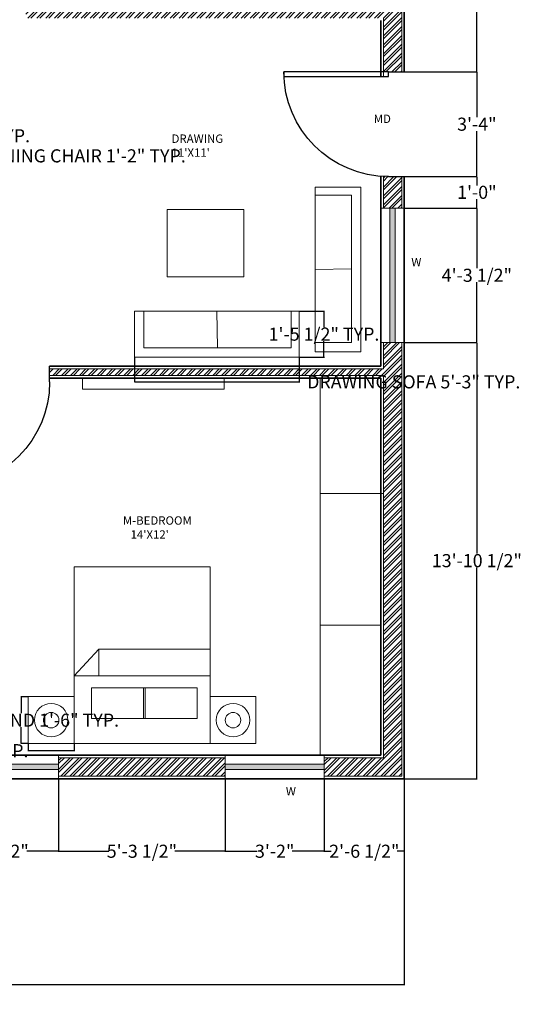
# Model space of a CAD drawing. Units: inches. Extents: x -340 to 394, y 381 to 1380.
# Tile 2 of 3: x 195 to 386, y 381 to 757. Entities that reach past the tile are written whole.
import ezdxf

# ---------------------------------------------------------------- set-up
doc = ezdxf.new("R2010")
doc.units = ezdxf.units.IN
doc.header["$MEASUREMENT"] = 0
for name, color, linetype, lineweight in [('A-ANNO-DIMS', 150, 'Continuous', 18), ('A-ANNO-TEXT', 11, 'Continuous', 18), ('A-AREA-IDEN', 11, 'Continuous', 18), ('A-FLOR-CASE', 130, 'Continuous', 20), ('A-GLAZ-PATT', 220, 'Continuous', 13), ('A-WALL-FNSH', 150, 'Continuous', 18), ('A-WALL-PATT', 10, 'Continuous', 13), ('door', 200, 'Continuous', 25), ('fur', 130, 'Continuous', 18), ('wall', 150, 'Continuous', 35), ('wind', 220, 'Continuous', 20)]:
    doc.layers.add(name, color=color, linetype=linetype, lineweight=lineweight)
doc.styles.get("Standard").update_dxf_attribs({"font": 'arial.ttf'})
doc.dimstyles.get("Standard").update_dxf_attribs({"dimtxt": 5, "dimasz": 0.18, "dimexe": 0.18, "dimexo": 0.0625, "dimgap": 0.09, "dimtad": 0, "dimtih": 1, "dimtoh": 1, "dimdec": 0, "dimzin": 0, "dimdsep": 46, "dimlunit": 4, "dimtxsty": 'Standard', "dimcen": 0.09, "dimadec": 0, "dimazin": 0, "dimtfac": 1, "dimtdec": 0, "dimtofl": 0, "dimtmove": 0, "dimatfit": 3, "dimfxl": 1, "dimtolj": 1, "dimtzin": 0, "dimarcsym": 0})

# ---------------------------------------------------------------- blocks, each defined once
blk = doc.blocks.new('*U2')
for p, q in [((0, 0), (0, -6)), ((40, 0), (40, -6))]:
    blk.add_line(p, q)
blk.add_lwpolyline([(0, 0), (0, 40), (1.75, 40), (1.75, 0)], close=True)
blk.add_arc((0, 0), 40, 0, 90)
blk = doc.blocks.new('BED-DOUBLE')
for p, q in [((25.93, 0), (25.93, 51.94)), ((25.93, 51.94), (25.93, 42.46)), ((36.06, 42.46), (25.93, 51.94)), ((25.93, 51.94), (36.06, 42.46)), ((25.93, 42.46), (36.06, 42.46)), ((36.06, 42.46), (36.06, 0))]:
    blk.add_line(p, q)
for points in [[(0, 0), (67.52, 0), (67.52, 51.94), (0, 51.94)], [(9.57, 24.81), (21.34, 24.81), (21.34, 45.28), (9.57, 45.28)], [(9.57, 4.93), (21.34, 4.93), (21.34, 25.4), (9.57, 25.4)]]:
    blk.add_lwpolyline(points, close=True)
blk = doc.blocks.new('NIGHTSTAND')
blk.add_lwpolyline([(0, 0), (17.94, 0), (17.94, 17.5), (0, 17.5)], close=True)
for radius in [6.39, 2.96]:
    blk.add_circle((8.97, 8.75), radius)
blk = doc.blocks.new('SOFA-DRAWING-ROOM')
for p, q in [((3.53, 17.55), (3.53, 3.6)), ((31.47, 17.55), (31.68, 3.6)), ((59.83, 3.6), (59.83, 17.55)), ((3.53, 3.6), (59.83, 3.6))]:
    blk.add_line(p, q)
blk.add_lwpolyline([(0, 0), (62.94, 0), (62.94, 17.55), (0, 17.55)], close=True)
blk = doc.blocks.new('*D13')
at = {"layer": 'A-ANNO-DIMS', "color": 0, "lineweight": -2, "transparency": 16777216}
for p, q in [((197.74, 498.52), (194.94, 498.52)), ((195.12, 498.34), (195.12, 492.23)), ((195.12, 480.77), (195.12, 486.88)), ((197.74, 480.59), (194.94, 480.59))]:
    blk.add_line(p, q, dxfattribs=at)
at = {"layer": 'A-ANNO-DIMS', "color": 0, "transparency": 16777216}
for points in [[(195.09, 498.34), (195.15, 498.34), (195.12, 498.52)], [(195.09, 480.77), (195.15, 480.77), (195.12, 480.59)]]:
    blk.add_solid(points, dxfattribs=at)
at = {"layer": 'Defpoints', "color": 0, "transparency": 16777216}
for p in [(195.12, 498.52), (197.81, 498.52), (197.81, 480.59)]:
    blk.add_point(p, dxfattribs=at)
at = {"layer": 'A-ANNO-DIMS', "color": 0, "transparency": 16777216, "insert": (195.12, 489.55), "char_height": 5, "attachment_point": 5}
blk.add_mtext('\\A1;NIGHTSTAND 1\'-6" TYP.', dxfattribs=at)
blk = doc.blocks.new('*D14')
at = {"layer": 'A-ANNO-DIMS', "color": 0, "lineweight": -2, "transparency": 16777216}
for p, q in [((197.81, 477.9), (197.63, 477.9)), ((197.81, 480.52), (197.81, 477.72)), ((215.12, 477.9), (197.99, 477.9)), ((215.3, 480.52), (215.3, 477.72))]:
    blk.add_line(p, q, dxfattribs=at)
at = {"layer": 'A-ANNO-DIMS', "color": 0, "transparency": 16777216}
for points in [[(197.99, 477.93), (197.99, 477.87), (197.81, 477.9)], [(215.12, 477.93), (215.12, 477.87), (215.3, 477.9)]]:
    blk.add_solid(points, dxfattribs=at)
at = {"layer": 'Defpoints', "color": 0, "transparency": 16777216}
for p in [(197.81, 480.59), (197.81, 477.9), (215.3, 480.59)]:
    blk.add_point(p, dxfattribs=at)
at = {"layer": 'A-ANNO-DIMS', "color": 0, "transparency": 16777216, "insert": (176.71, 477.9), "char_height": 5, "attachment_point": 5}
blk.add_mtext('\\A1;1\'-5 1/2" TYP.', dxfattribs=at)
blk = doc.blocks.new('*D21')
at = {"layer": 'A-ANNO-DIMS', "color": 0, "lineweight": -2, "transparency": 16777216}
for p, q in [((238.33, 628.13), (238.33, 618.57)), ((301.27, 628.13), (301.27, 618.57)), ((238.51, 618.75), (301.09, 618.75)), ((301.27, 618.75), (301.45, 618.75))]:
    blk.add_line(p, q, dxfattribs=at)
at = {"layer": 'A-ANNO-DIMS', "color": 0, "transparency": 16777216}
for points in [[(238.51, 618.78), (238.51, 618.72), (238.33, 618.75)], [(301.09, 618.78), (301.09, 618.72), (301.27, 618.75)]]:
    blk.add_solid(points, dxfattribs=at)
at = {"layer": 'Defpoints', "color": 0, "transparency": 16777216}
for p in [(238.33, 628.19), (301.27, 628.19), (301.27, 618.75)]:
    blk.add_point(p, dxfattribs=at)
at = {"layer": 'A-ANNO-DIMS', "color": 0, "transparency": 16777216, "insert": (344.98, 618.75), "char_height": 5, "attachment_point": 5}
blk.add_mtext('\\A1;DRAWING SOFA 5\'-3" TYP.', dxfattribs=at)
blk = doc.blocks.new('*D22')
at = {"layer": 'A-ANNO-DIMS', "color": 0, "lineweight": -2, "transparency": 16777216}
for p, q in [((301.33, 645.74), (310.89, 645.74)), ((310.71, 645.56), (310.71, 639.64)), ((310.71, 628.37), (310.71, 634.29)), ((301.33, 628.19), (310.89, 628.19))]:
    blk.add_line(p, q, dxfattribs=at)
at = {"layer": 'A-ANNO-DIMS', "color": 0, "transparency": 16777216}
for points in [[(310.68, 645.56), (310.74, 645.56), (310.71, 645.74)], [(310.68, 628.37), (310.74, 628.37), (310.71, 628.19)]]:
    blk.add_solid(points, dxfattribs=at)
at = {"layer": 'Defpoints', "color": 0, "transparency": 16777216}
for p in [(301.27, 645.74), (310.71, 645.74), (301.27, 628.19)]:
    blk.add_point(p, dxfattribs=at)
at = {"layer": 'A-ANNO-DIMS', "color": 0, "transparency": 16777216, "insert": (310.71, 636.97), "char_height": 5, "attachment_point": 5}
blk.add_mtext('\\A1;1\'-5 1/2" TYP.', dxfattribs=at)
blk = doc.blocks.new('*D23')
at = {"layer": 'A-ANNO-DIMS', "color": 0, "lineweight": -2, "transparency": 16777216}
for p, q in [((165.2, 707.1), (165.2, 704.88)), ((179.21, 707.1), (179.21, 704.88)), ((165.38, 705.06), (179.03, 705.06)), ((179.21, 705.06), (179.39, 705.06))]:
    blk.add_line(p, q, dxfattribs=at)
at = {"layer": 'A-ANNO-DIMS', "color": 0, "transparency": 16777216}
for points in [[(165.38, 705.09), (165.38, 705.03), (165.2, 705.06)], [(179.03, 705.09), (179.03, 705.03), (179.21, 705.06)]]:
    blk.add_solid(points, dxfattribs=at)
at = {"layer": 'Defpoints', "color": 0, "transparency": 16777216}
for p in [(165.2, 707.16), (179.21, 707.16), (179.21, 705.06)]:
    blk.add_point(p, dxfattribs=at)
at = {"layer": 'A-ANNO-DIMS', "color": 0, "transparency": 16777216, "insert": (219.63, 705.06), "char_height": 5, "attachment_point": 5}
blk.add_mtext('\\A1;DINING CHAIR 1\'-2" TYP.', dxfattribs=at)
blk = doc.blocks.new('*D24')
at = {"layer": 'A-ANNO-DIMS', "color": 0, "lineweight": -2, "transparency": 16777216}
for p, q in [((179.28, 718.31), (181.5, 718.31)), ((181.32, 718.13), (181.32, 715.38)), ((179.28, 707.16), (181.5, 707.16)), ((181.32, 707.34), (181.32, 710.09))]:
    blk.add_line(p, q, dxfattribs=at)
at = {"layer": 'A-ANNO-DIMS', "color": 0, "transparency": 16777216}
for points in [[(181.29, 718.13), (181.35, 718.13), (181.32, 718.31)], [(181.29, 707.34), (181.35, 707.34), (181.32, 707.16)]]:
    blk.add_solid(points, dxfattribs=at)
at = {"layer": 'Defpoints', "color": 0, "transparency": 16777216}
for p in [(179.21, 718.31), (181.32, 718.31), (179.21, 707.16)]:
    blk.add_point(p, dxfattribs=at)
at = {"layer": 'A-ANNO-DIMS', "color": 0, "transparency": 16777216, "insert": (181.32, 712.74), "char_height": 5, "attachment_point": 5}
blk.add_mtext('\\A1;0\'-11" TYP.', dxfattribs=at)
blk = doc.blocks.new('*D25')
at = {"layer": 'A-ANNO-DIMS', "color": 0, "lineweight": -2, "transparency": 16777216}
for p, q in [((341.44, 633.76), (369.26, 633.76)), ((369.08, 633.58), (369.08, 553.16)), ((369.08, 467.38), (369.08, 547.8)), ((341.44, 467.2), (369.26, 467.2))]:
    blk.add_line(p, q, dxfattribs=at)
at = {"layer": 'A-ANNO-DIMS', "color": 0, "transparency": 16777216}
for points in [[(369.05, 633.58), (369.11, 633.58), (369.08, 633.76)], [(369.05, 467.38), (369.11, 467.38), (369.08, 467.2)]]:
    blk.add_solid(points, dxfattribs=at)
at = {"layer": 'Defpoints', "color": 0, "transparency": 16777216}
for p in [(341.38, 633.76), (369.08, 633.76), (341.38, 467.2)]:
    blk.add_point(p, dxfattribs=at)
at = {"layer": 'A-ANNO-DIMS', "color": 0, "transparency": 16777216, "insert": (369.08, 550.48), "char_height": 5, "attachment_point": 5}
blk.add_mtext('\\A1;13\'-10 1/2"', dxfattribs=at)
blk = doc.blocks.new('*D26')
at = {"layer": 'A-ANNO-DIMS', "color": 0, "lineweight": -2, "transparency": 16777216}
for p, q in [((341.44, 685.13), (369.26, 685.13)), ((369.08, 684.95), (369.08, 662.12)), ((369.08, 633.94), (369.08, 656.77)), ((341.44, 633.76), (369.26, 633.76))]:
    blk.add_line(p, q, dxfattribs=at)
at = {"layer": 'A-ANNO-DIMS', "color": 0, "transparency": 16777216}
for points in [[(369.05, 684.95), (369.11, 684.95), (369.08, 685.13)], [(369.05, 633.94), (369.11, 633.94), (369.08, 633.76)]]:
    blk.add_solid(points, dxfattribs=at)
at = {"layer": 'Defpoints', "color": 0, "transparency": 16777216}
for p in [(341.38, 685.13), (369.08, 685.13), (341.38, 633.76)]:
    blk.add_point(p, dxfattribs=at)
at = {"layer": 'A-ANNO-DIMS', "color": 0, "transparency": 16777216, "insert": (369.08, 659.45), "char_height": 5, "attachment_point": 5}
blk.add_mtext('\\A1;4\'-3 1/2"', dxfattribs=at)
blk = doc.blocks.new('*D27')
at = {"layer": 'A-ANNO-DIMS', "color": 0, "lineweight": -2, "transparency": 16777216}
for p, q in [((341.44, 697.15), (369.26, 697.15)), ((369.08, 696.97), (369.08, 693.78)), ((369.08, 685.31), (369.08, 688.49)), ((341.44, 685.13), (369.26, 685.13))]:
    blk.add_line(p, q, dxfattribs=at)
at = {"layer": 'A-ANNO-DIMS', "color": 0, "transparency": 16777216}
for points in [[(369.05, 696.97), (369.11, 696.97), (369.08, 697.15)], [(369.05, 685.31), (369.11, 685.31), (369.08, 685.13)]]:
    blk.add_solid(points, dxfattribs=at)
at = {"layer": 'Defpoints', "color": 0, "transparency": 16777216}
for p in [(341.38, 697.15), (369.08, 697.15), (341.38, 685.13)]:
    blk.add_point(p, dxfattribs=at)
at = {"layer": 'A-ANNO-DIMS', "color": 0, "transparency": 16777216, "insert": (369.08, 691.14), "char_height": 5, "attachment_point": 5}
blk.add_mtext('\\A1;1\'-0"', dxfattribs=at)
blk = doc.blocks.new('*D28')
at = {"layer": 'A-ANNO-DIMS', "color": 0, "lineweight": -2, "transparency": 16777216}
for p, q in [((341.44, 737.15), (369.26, 737.15)), ((369.08, 736.97), (369.08, 719.79)), ((369.08, 697.33), (369.08, 714.5)), ((341.44, 697.15), (369.26, 697.15))]:
    blk.add_line(p, q, dxfattribs=at)
at = {"layer": 'A-ANNO-DIMS', "color": 0, "transparency": 16777216}
for points in [[(369.05, 736.97), (369.11, 736.97), (369.08, 737.15)], [(369.05, 697.33), (369.11, 697.33), (369.08, 697.15)]]:
    blk.add_solid(points, dxfattribs=at)
at = {"layer": 'Defpoints', "color": 0, "transparency": 16777216}
for p in [(341.38, 737.15), (369.08, 737.15), (341.38, 697.15)]:
    blk.add_point(p, dxfattribs=at)
at = {"layer": 'A-ANNO-DIMS', "color": 0, "transparency": 16777216, "insert": (369.08, 717.15), "char_height": 5, "attachment_point": 5}
blk.add_mtext('\\A1;3\'-4"', dxfattribs=at)
blk = doc.blocks.new('*D29')
at = {"layer": 'A-ANNO-DIMS', "color": 0, "lineweight": -2, "transparency": 16777216}
for p, q in [((341.44, 801.11), (369.26, 801.11)), ((369.08, 800.93), (369.08, 771.76)), ((369.08, 737.33), (369.08, 766.49)), ((341.44, 737.15), (369.26, 737.15))]:
    blk.add_line(p, q, dxfattribs=at)
at = {"layer": 'A-ANNO-DIMS', "color": 0, "transparency": 16777216}
for points in [[(369.05, 800.93), (369.11, 800.93), (369.08, 801.11)], [(369.05, 737.33), (369.11, 737.33), (369.08, 737.15)]]:
    blk.add_solid(points, dxfattribs=at)
at = {"layer": 'Defpoints', "color": 0, "transparency": 16777216}
for p in [(341.38, 801.11), (369.08, 801.11), (341.38, 737.15)]:
    blk.add_point(p, dxfattribs=at)
at = {"layer": 'A-ANNO-DIMS', "color": 0, "transparency": 16777216, "insert": (369.08, 769.13), "char_height": 5, "attachment_point": 5}
blk.add_mtext('\\A1;5\'-4"', dxfattribs=at)
blk = doc.blocks.new('*D54')
at = {"layer": 'A-ANNO-DIMS', "color": 0, "lineweight": -2, "transparency": 16777216}
for p, q in [((171.54, 467.14), (171.54, 439.32)), ((209.39, 467.14), (209.39, 439.32)), ((171.72, 439.5), (183.73, 439.5)), ((209.21, 439.5), (197.2, 439.5))]:
    blk.add_line(p, q, dxfattribs=at)
at = {"layer": 'A-ANNO-DIMS', "color": 0, "transparency": 16777216}
for points in [[(171.72, 439.53), (171.72, 439.47), (171.54, 439.5)], [(209.21, 439.53), (209.21, 439.47), (209.39, 439.5)]]:
    blk.add_solid(points, dxfattribs=at)
at = {"layer": 'Defpoints', "color": 0, "transparency": 16777216}
for p in [(171.54, 467.2), (209.39, 467.2), (171.54, 439.5)]:
    blk.add_point(p, dxfattribs=at)
at = {"layer": 'A-ANNO-DIMS', "color": 0, "transparency": 16777216, "insert": (190.47, 439.5), "char_height": 5, "attachment_point": 5}
blk.add_mtext('\\A1;3\'-2"', dxfattribs=at)
blk = doc.blocks.new('*D55')
at = {"layer": 'A-ANNO-DIMS', "color": 0, "lineweight": -2, "transparency": 16777216}
for p, q in [((209.39, 467.14), (209.39, 439.32)), ((272.96, 467.14), (272.96, 439.32)), ((209.57, 439.5), (228.62, 439.5)), ((272.78, 439.5), (253.74, 439.5))]:
    blk.add_line(p, q, dxfattribs=at)
at = {"layer": 'A-ANNO-DIMS', "color": 0, "transparency": 16777216}
for points in [[(209.57, 439.53), (209.57, 439.47), (209.39, 439.5)], [(272.78, 439.53), (272.78, 439.47), (272.96, 439.5)]]:
    blk.add_solid(points, dxfattribs=at)
at = {"layer": 'Defpoints', "color": 0, "transparency": 16777216}
for p in [(209.39, 467.2), (272.96, 467.2), (209.39, 439.5)]:
    blk.add_point(p, dxfattribs=at)
at = {"layer": 'A-ANNO-DIMS', "color": 0, "transparency": 16777216, "insert": (241.18, 439.5), "char_height": 5, "attachment_point": 5}
blk.add_mtext('\\A1;5\'-3 1/2"', dxfattribs=at)
blk = doc.blocks.new('*D56')
at = {"layer": 'A-ANNO-DIMS', "color": 0, "lineweight": -2, "transparency": 16777216}
for p, q in [((272.96, 467.14), (272.96, 439.32)), ((310.81, 467.14), (310.81, 439.32)), ((273.14, 439.5), (285.15, 439.5)), ((310.63, 439.5), (298.62, 439.5))]:
    blk.add_line(p, q, dxfattribs=at)
at = {"layer": 'A-ANNO-DIMS', "color": 0, "transparency": 16777216}
for points in [[(273.14, 439.53), (273.14, 439.47), (272.96, 439.5)], [(310.63, 439.53), (310.63, 439.47), (310.81, 439.5)]]:
    blk.add_solid(points, dxfattribs=at)
at = {"layer": 'Defpoints', "color": 0, "transparency": 16777216}
for p in [(272.96, 467.2), (310.81, 467.2), (272.96, 439.5)]:
    blk.add_point(p, dxfattribs=at)
at = {"layer": 'A-ANNO-DIMS', "color": 0, "transparency": 16777216, "insert": (291.89, 439.5), "char_height": 5, "attachment_point": 5}
blk.add_mtext('\\A1;3\'-2"', dxfattribs=at)
blk = doc.blocks.new('*D57')
at = {"layer": 'A-ANNO-DIMS', "color": 0, "lineweight": -2, "transparency": 16777216}
for p, q in [((310.81, 467.14), (310.81, 439.32)), ((341.38, 467.14), (341.38, 439.32)), ((310.99, 439.5), (313.49, 439.5)), ((341.2, 439.5), (338.7, 439.5))]:
    blk.add_line(p, q, dxfattribs=at)
at = {"layer": 'A-ANNO-DIMS', "color": 0, "transparency": 16777216}
for points in [[(310.99, 439.53), (310.99, 439.47), (310.81, 439.5)], [(341.2, 439.53), (341.2, 439.47), (341.38, 439.5)]]:
    blk.add_solid(points, dxfattribs=at)
at = {"layer": 'Defpoints', "color": 0, "transparency": 16777216}
for p in [(310.81, 467.2), (341.38, 467.2), (310.81, 439.5)]:
    blk.add_point(p, dxfattribs=at)
at = {"layer": 'A-ANNO-DIMS', "color": 0, "transparency": 16777216, "insert": (326.1, 439.5), "char_height": 5, "attachment_point": 5}
blk.add_mtext('\\A1;2\'-6 1/2"', dxfattribs=at)
blk = doc.blocks.new('*D58')
at = {"layer": 'A-ANNO-DIMS', "color": 0, "lineweight": -2, "transparency": 16777216}
for p, q in [((-64.94, 620.44), (-64.94, 388.32)), ((341.38, 467.14), (341.38, 388.32)), ((-64.76, 388.5), (121.78, 388.5)), ((341.2, 388.5), (154.67, 388.5))]:
    blk.add_line(p, q, dxfattribs=at)
at = {"layer": 'A-ANNO-DIMS', "color": 0, "transparency": 16777216}
for points in [[(-64.76, 388.53), (-64.76, 388.47), (-64.94, 388.5)], [(341.2, 388.53), (341.2, 388.47), (341.38, 388.5)]]:
    blk.add_solid(points, dxfattribs=at)
at = {"layer": 'Defpoints', "color": 0, "transparency": 16777216}
for p in [(-64.94, 620.5), (341.38, 467.2), (341.38, 388.5)]:
    blk.add_point(p, dxfattribs=at)
at = {"layer": 'A-ANNO-DIMS', "color": 0, "transparency": 16777216, "insert": (138.22, 388.5), "char_height": 5, "attachment_point": 5}
blk.add_mtext('\\A1;33\'-10 1/2"', dxfattribs=at)

msp = doc.modelspace()

# ---------------------------------------------------------------- hatches: boundary and pattern name
at = {"layer": 'A-GLAZ-PATT'}
h = msp.add_hatch(color=256, dxfattribs=at)
h.dxf.hatch_style = 1
h.paths.add_polyline_path([(58.56, 910.7), (-1.68, 910.7), (-1.68, 908.7), (58.56, 908.7)])
h.paths.add_polyline_path([(115.02, 910.7), (93.88, 910.7), (93.88, 908.7), (115.02, 908.7)])
h.paths.add_polyline_path([(206.8, 910.7), (185.67, 910.7), (185.67, 908.7), (206.8, 908.7)])
h.paths.add_polyline_path([(308.48, 910.7), (236.12, 910.7), (236.12, 908.7), (308.48, 908.7)])
h.paths.add_polyline_path([(337.88, 852.47), (335.88, 852.47), (335.88, 801.11), (337.88, 801.11)])
h.paths.add_polyline_path([(-34.12, 843.05), (-36.12, 843.05), (-36.12, 791.69), (-34.12, 791.69)])
h.paths.add_polyline_path([(-0.92, 737.98), (-2.92, 737.98), (-2.92, 646.31), (-0.92, 646.31)])
h.paths.add_polyline_path([(337.88, 685.13), (335.88, 685.13), (335.88, 633.76), (337.88, 633.76)])
h.paths.add_polyline_path([(19, 527.45), (-19.67, 527.45), (-19.67, 525.45), (19, 525.45)])
h.paths.add_polyline_path([(63.15, 472.7), (2.91, 472.7), (2.91, 470.7), (63.15, 470.7)])
h.paths.add_polyline_path([(121.02, 472.7), (99.88, 472.7), (99.88, 470.7), (121.02, 470.7)])
h.paths.add_polyline_path([(310.81, 472.7), (272.96, 472.7), (272.96, 470.7), (310.81, 470.7)])
h.paths.add_polyline_path([(209.39, 472.7), (171.54, 472.7), (171.54, 470.7), (209.39, 470.7)])
at = {"layer": 'A-WALL-PATT'}
h = msp.add_hatch(dxfattribs=at)
h.set_pattern_fill('ANSI32', color=256, scale=6.4)
h.paths.add_polyline_path([(211.38, 905.2), (208.88, 905.2), (208.88, 859.96), (211.38, 859.96)])
h.paths.add_polyline_path([(211.38, 833.2), (208.88, 833.2), (208.88, 808.2), (146.36, 808.2), (146.36, 805.7), (211.38, 805.7)])
h.paths.add_polyline_path([(92.88, 905.2), (90.38, 905.2), (90.38, 805.7), (119.27, 805.7), (119.27, 808.2), (92.88, 808.2)])
h.paths.add_polyline_path([(1.58, 756.7), (-5.42, 756.7), (-5.42, 737.98), (1.58, 737.98)], flags=17)
h.paths.add_polyline_path([(1.58, 646.31), (-5.42, 646.31), (-5.42, 629.2), (1.58, 629.2)])
h.paths.add_polyline_path([(340.38, 697.15), (335.38, 697.15, -0.012506), (333.38, 697.2), (333.38, 685.13), (340.38, 685.13)])
h.paths.add_polyline_path([(29.76, 527.7), (19, 527.7), (19, 525.2), (29.76, 525.2)], flags=17)
h.paths.add_polyline_path([(98.88, 579.2), (160.88, 579.2), (160.88, 548.2), (161.03, 548.2), (163.38, 548.2), (163.38, 621.2), (165.94, 621.2), (165.94, 623.7), (160.88, 623.7), (160.88, 581.7), (96.38, 581.7), (96.38, 527.7), (69.71, 527.7), (69.71, 525.2), (96.38, 525.2), (96.38, 475.2), (63.15, 475.2), (63.15, 468.2), (98.88, 468.2)])
h.paths.add_polyline_path([(171.54, 475.2), (163.38, 475.2), (163.38, 525.87), (160.88, 525.87), (160.88, 475.2), (121.02, 475.2), (121.02, 468.2), (159.88, 468.2), (171.54, 468.2)])
h.paths.add_polyline_path([(272.96, 475.2), (209.39, 475.2), (209.39, 468.2), (272.96, 468.2)], flags=17)
h.paths.add_polyline_path([(340.38, 620.2), (340.38, 633.76), (333.38, 633.76), (333.38, 623.7), (205.94, 623.7), (205.94, 621.2), (333.38, 621.2), (333.38, 475.2), (310.81, 475.2), (310.81, 468.2), (340.38, 468.2)])
h = msp.add_hatch(dxfattribs=at)
h.set_pattern_fill('ANSI32', color=256, scale=6.4)
h.paths.add_polyline_path([(116.88, 628.2), (-38.62, 628.2), (-38.62, 528.7), (-38.62, 468.2), (2.91, 468.2), (2.91, 475.2), (-31.62, 475.2), (-31.62, 525.2), (-19.67, 525.2), (-19.67, 527.7), (-31.62, 527.7), (-31.62, 625.7), (114.38, 625.7), (114.38, 624.7), (116.88, 624.7)])
h.paths.add_polyline_path([(-31.62, 791.69), (-38.62, 791.69), (-38.62, 757.7), (89.38, 757.7), (89.38, 760.2), (-31.62, 760.2)])
h.paths.add_polyline_path([(340.38, 801.11), (333.38, 801.11), (333.38, 760.2), (332.38, 760.2), (196.87, 760.2), (196.87, 757.7), (332.38, 757.7), (333.38, 757.7), (333.38, 746.4), (333.38, 737.15), (335.38, 737.15), (340.38, 737.15), (340.38, 756.7)])

# ---------------------------------------------------------------- linework, layer by layer
at = {"layer": 'A-FLOR-CASE'}
for p, q in [((309.22, 620.2), (309.22, 476.2)), ((309.22, 576.09), (333.38, 576.09)), ((309.22, 525.86), (332.38, 525.86))]:
    msp.add_line(p, q, dxfattribs=at)
at = {"layer": 'A-WALL-FNSH'}
for p, q in [((340.38, 801.11), (340.38, 756.7)), ((333.38, 746.4), (333.38, 757.7)), ((333.38, 756.7), (333.38, 735.4)), ((340.38, 756.7), (340.38, 737.15)), ((333.38, 697.2), (333.38, 685.13)), ((340.38, 697.15), (340.38, 685.13)), ((333.38, 633.76), (333.38, 623.7)), ((340.38, 633.76), (340.38, 620.2)), ((333.38, 623.7), (205.94, 623.7)), ((333.38, 621.2), (205.94, 621.2)), ((333.38, 621.2), (333.38, 475.2)), ((340.38, 620.2), (340.38, 468.2)), ((272.96, 475.2), (209.39, 475.2)), ((333.38, 475.2), (310.81, 475.2)), ((272.96, 468.2), (209.39, 468.2)), ((340.38, 468.2), (310.81, 468.2))]:
    msp.add_line(p, q, dxfattribs=at)
at = {"layer": 'fur'}
for points in [[(280.15, 684.61), (250.79, 684.61), (250.79, 658.8), (280.15, 658.8)], [(218.56, 620.2), (272.63, 620.2), (272.63, 615.96), (218.56, 615.96)]]:
    msp.add_lwpolyline(points, close=True, dxfattribs=at)
at = {"layer": 'wall'}
for p, q in [((341.38, 914.2), (341.38, 756.7)), ((341.38, 737.15), (341.38, 801.11)), ((332.38, 756.7), (332.38, 735.4)), ((332.38, 756.7), (332.38, 737.15)), ((341.38, 756.7), (341.38, 737.15)), ((332.38, 697.26), (332.38, 624.7)), ((332.38, 697.26), (332.38, 685.13)), ((341.38, 697.15), (341.38, 620.2)), ((341.38, 697.15), (341.38, 685.13)), ((332.38, 633.76), (332.38, 624.7)), ((341.38, 467.2), (341.38, 633.76)), ((332.38, 624.7), (205.94, 624.7)), ((332.38, 624.7), (205.94, 624.7)), ((332.38, 620.2), (205.94, 620.2)), ((205.94, 620.2), (332.38, 620.2)), ((332.38, 620.2), (332.38, 476.2)), ((332.38, 620.2), (332.38, 476.2)), ((341.38, 620.2), (341.38, 467.2)), ((332.38, 476.2), (164.38, 476.2)), ((209.39, 476.2), (272.96, 476.2)), ((332.38, 476.2), (310.81, 476.2)), ((341.38, 467.2), (159.88, 467.2)), ((272.96, 467.2), (209.39, 467.2)), ((310.81, 467.2), (341.38, 467.2))]:
    msp.add_line(p, q, dxfattribs=at)
at = {"layer": 'wind'}
for p, q in [((335.88, 633.76), (335.88, 685.13)), ((337.88, 633.76), (337.88, 685.13)), ((171.54, 472.7), (209.39, 472.7)), ((171.54, 470.7), (209.39, 470.7)), ((272.96, 472.7), (310.81, 472.7)), ((272.96, 470.7), (310.81, 470.7))]:
    msp.add_line(p, q, dxfattribs=at)
for points in [[(332.38, 633.76), (341.38, 633.76), (341.38, 685.13), (332.38, 685.13)], [(171.54, 476.2), (209.39, 476.2), (209.39, 467.2), (171.54, 467.2)], [(272.96, 476.2), (310.81, 476.2), (310.81, 467.2), (272.96, 467.2)]]:
    msp.add_lwpolyline(points, close=True, dxfattribs=at)

# ---------------------------------------------------------------- block references
at = {"layer": 'door', "xscale": -1}
for p, rotation in [((335.38, 737.15), 90), ((165.94, 618.7), 180)]:
    msp.add_blockref('*U2', p, dxfattribs=dict(at, rotation=rotation))
at = {"layer": 'fur'}
for name, p, rotation in [('SOFA-DRAWING-ROOM', (324.83, 630.19), 90.0000000000004), ('BED-DOUBLE', (267.24, 480.59), 89.99999999999957), ('NIGHTSTAND', (215.3, 480.59), 90.00000000000018), ('NIGHTSTAND', (284.74, 480.59), 90)]:
    msp.add_blockref(name, p, dxfattribs=dict(at, rotation=rotation))
msp.add_blockref('SOFA-DRAWING-ROOM', (238.33, 628.19), dxfattribs=at)

# ---------------------------------------------------------------- texts
at = {"layer": 'A-ANNO-TEXT', "char_height": 3.2, "attachment_point": 1}
for s, insert in [('MD', (329.71, 720.8)), ('W', (344.06, 666.05)), ('W', (296.15, 463.99))]:
    msp.add_mtext_dynamic_manual_height_columns(s, width=932.3287, gutter_width=16, heights=[0], dxfattribs=dict(at, insert=insert))
at = {"layer": 'A-AREA-IDEN', "char_height": 3.2, "attachment_point": 1}
for s, insert in [("DRAWING\\P11'X11'", (252.51, 713.22)), ("M-BEDROOM\\P   14'X12'", (233.93, 567.4))]:
    msp.add_mtext_dynamic_manual_height_columns(s, width=932.3287, gutter_width=16, heights=[0], dxfattribs=dict(at, insert=insert))

# ---------------------------------------------------------------- dimensions: what is measured, and where the dimension line sits
at = {"layer": 'A-ANNO-DIMS'}
for base, p1, p2, angle, picture, middle in [((369.08, 801.11), (341.38, 737.15), (341.38, 801.11), 90, '*D29', (369.08, 769.13)), ((369.08, 737.15), (341.38, 697.15), (341.38, 737.15), 90, '*D28', (369.08, 717.15)), ((369.08, 697.15), (341.38, 685.13), (341.38, 697.15), 90, '*D27', (369.08, 691.14)), ((369.08, 685.13), (341.38, 633.76), (341.38, 685.13), 90, '*D26', (369.08, 659.45)), ((369.08, 633.76), (341.38, 467.2), (341.38, 633.76), 90, '*D25', (369.08, 550.48)), ((171.5386, 439.4996), (209.3945, 467.1996), (171.5386, 467.1996), 180, '*D54', (190.4665, 439.4996)), ((209.39, 439.5), (272.96, 467.2), (209.39, 467.2), 180, '*D55', (241.18, 439.5)), ((272.9585, 439.4996), (310.8143, 467.1996), (272.9585, 467.1996), 180, '*D56', (291.8864, 439.4996)), ((310.81, 439.5), (341.38, 467.2), (310.81, 467.2), 180, '*D57', (326.1, 439.5))]:
    dim = msp.add_linear_dim(base=base, p1=p1, p2=p2, angle=angle, dimstyle='Standard', override={"dimdec": 1, "dimlfac": 1, "dimrnd": 0, "dimzin": 1, "dimdsep": 46, "dimlunit": 4, "dimfrac": 2}, dxfattribs=at)
    dim.commit()
    dim.dimension.update_dxf_attribs({"geometry": picture, "text_midpoint": middle})
for base, p1, p2, angle, text, picture, middle in [((181.3151, 718.3112), (179.213, 707.161), (179.213, 718.3112), 90, '<> TYP.', '*D24', (181.3151, 712.7361)), ((310.7071, 645.7431), (301.2664, 628.1928), (301.2664, 645.7431), 90, '<> TYP.', '*D22', (310.7071, 636.9679)), ((195.12, 498.52), (197.81, 480.59), (197.81, 498.52), 90, 'NIGHTSTAND <> TYP.', '*D13', (195.12, 489.55)), ((197.81, 477.9), (215.3, 480.59), (197.81, 480.59), 180, '<> TYP.', '*D14', (176.71, 477.9))]:
    dim = msp.add_linear_dim(base=base, p1=p1, p2=p2, angle=angle, text=text, dimstyle='Standard', override={"dimdec": 1, "dimlfac": 1, "dimrnd": 0, "dimzin": 1, "dimdsep": 46, "dimlunit": 4, "dimfrac": 2}, dxfattribs=at)
    dim.commit()
    dim.dimension.update_dxf_attribs({"geometry": picture, "text_midpoint": middle})
for base, p1, p2, text, picture, middle in [((179.21, 705.06), (165.2, 707.16), (179.21, 707.16), 'DINING CHAIR <> TYP.', '*D23', (219.63, 705.06)), ((301.27, 618.75), (238.33, 628.19), (301.27, 628.19), 'DRAWING SOFA <> TYP.', '*D21', (344.98, 618.75))]:
    dim = msp.add_linear_dim(base=base, p1=p1, p2=p2, text=text, dimstyle='Standard', override={"dimdec": 1, "dimlfac": 1, "dimrnd": 0, "dimzin": 1, "dimdsep": 46, "dimlunit": 4, "dimfrac": 2}, dxfattribs=at)
    dim.commit()
    dim.dimension.update_dxf_attribs({"geometry": picture, "text_midpoint": middle})
dim = msp.add_linear_dim(base=(341.38, 388.5), p1=(-64.94, 620.5), p2=(341.38, 467.2), dimstyle='Standard', override={"dimdec": 1, "dimlfac": 1, "dimrnd": 0, "dimzin": 1, "dimdsep": 46, "dimlunit": 4, "dimfrac": 2}, dxfattribs=at)
dim.commit()
dim.dimension.update_dxf_attribs({"geometry": '*D58', "text_midpoint": (138.22, 388.5)})

doc.saveas('drawing.dxf')
